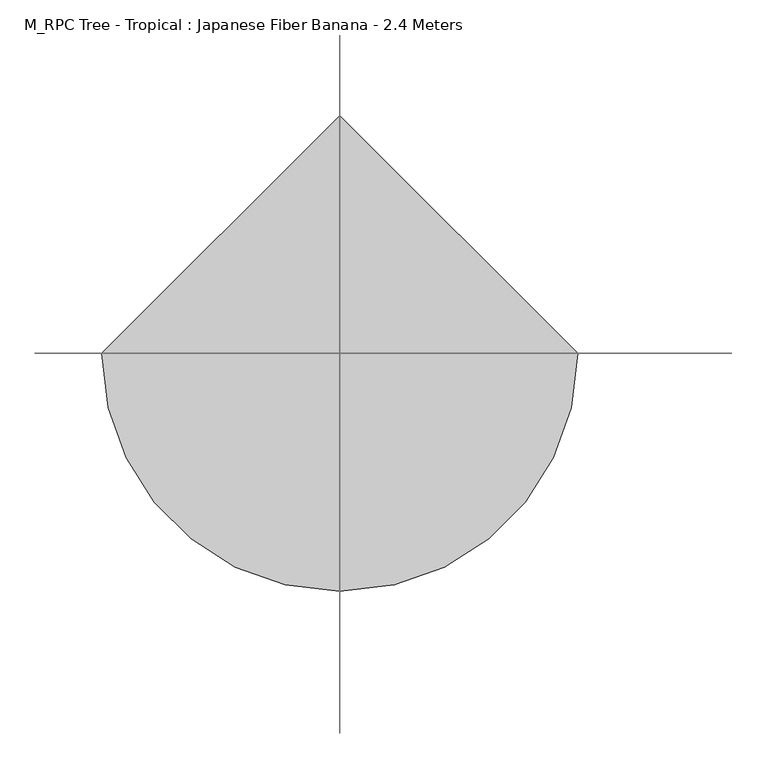
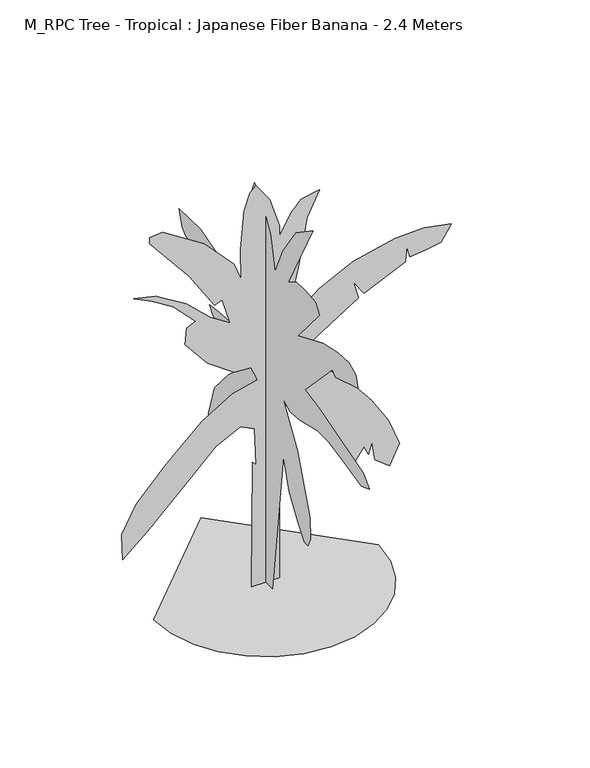
"""IFC4 building model written with IfcOpenShell, lengths in millimetres: geographic element geometry, M_RPC Tree - Tropical : Japanese Fiber Banana - 2.4 Meters."""

from ifc_helpers import new_model, si_unit, origin, place, context, project, spatial, triangles, source, transform, mapped, element, save


def m_rpc_tree_tropical_japanese_fiber_banana_2_4_meters_2e6d15ad(model_context):
    return source(origin(), model_context, "Body", "Tessellation", [
        triangles([(-639.3178808, 0.0, 3.7e-06), (-622.4128807, -146.5347148, 3.7e-06), (-574.2626584, -281.1033905, 3.7e-06), (-498.7249, -399.8512839, 3.7e-06), (-399.6546026, -498.9215813, 3.7e-06), (-280.9067273, -574.4593397, 3.7e-06), (-146.3380426, -622.6095257, 3.7e-06), (0.196699, -639.5145258, 3.7e-06), (146.7313871, -622.6095257, 3.7e-06), (281.3000536, -574.4593397, 3.7e-06), (400.0479652, -498.9215813, 3.7e-06), (499.1182626, -399.8512839, 3.7e-06), (574.656021, -281.1033905, 3.7e-06), (622.8061707, -146.5344696, 3.7e-06), (639.7111708, 5.59e-05, 3.7e-06), (0.1965872, 639.5145258, 3.7e-06), (72.5559047, -2.4e-06, 1465.492234), (85.0391952, -3.9e-06, 1478.3097656), (106.8852636, -6.2e-06, 1497.8148251), (136.5331088, -9.2e-06, 1522.8923641), (172.4227059, -1.28e-05, 1552.4299507), (212.9935943, -1.67e-05, 1585.3100658), (256.6849863, -2.09e-05, 1620.4176613), (301.9376202, -2.52e-05, 1656.6427757), (497.3357769, -3.68e-05, 1754.3430622), (735.2139896, -4.34e-05, 1809.5632381), (900.8770609, -4.39e-05, 1813.8107986), (1053.7975233, -4.04e-05, 1784.075695), (994.3298595, -2.97e-05, 1694.872855), (909.3720366, -2.77e-05, 1677.8804329), (820.1692692, -2.67e-05, 1669.3853119), (803.1767017, -3.43e-05, 1733.1030796), (794.6816534, -2.42e-05, 1648.1478001), (556.8059478, -1.15e-05, 1541.9523926), (497.3357769, -2.16e-05, 1626.9076721), (527.0708805, -9.5e-06, 1524.9598251), (246.7159545, 1.13e-05, 1350.8018509), (204.2378242, 1.99e-05, 1278.5891075), (450.610613, 4.47e-05, 1070.4459257), (599.2835876, 6.7e-05, 883.5427992), (696.9839104, 8.52e-05, 730.6223368), (760.699062, 0.0001045, 569.2043189), (701.2313982, 0.0001181, 454.5139721), (620.5211357, 0.0001105, 518.2316671), (603.5311117, 9.74e-05, 628.6744898), (582.2910564, 0.000105, 564.9567947), (556.8059478, 9.84e-05, 620.1795141), (510.0808202, 0.0001065, 552.2142586), (233.9724192, 6.75e-05, 879.2953114), (98.0427347, 4.83e-05, 1040.7108221), (81.0516842, 4.01e-05, 1108.6760777), (76.8036695, 0.0001723, 0.0), (-80.3648348, 0.0001723, 0.0), (-76.1170745, 8.32e-05, 747.6123608), (-54.8780048, 8.57e-05, 726.3748489), (-63.3737798, 5.99e-05, 943.0130064), (-144.0820393, 5.48e-05, 985.4906462), (-284.259248, 6.29e-05, 917.5254633), (-492.4023934, 8.72e-05, 713.6297693), (-675.0579958, 0.000108, 539.4717224), (-815.2334513, 0.0001222, 420.5313443), (-819.4834826, 0.000104, 573.4543502), (-738.7732201, 8.57e-05, 726.3748489), (-564.6151368, 6.39e-05, 909.030415), (-364.9670033, 4.22e-05, 1091.685981), (-190.8077029, 2.95e-05, 1197.878845), (-46.382475, 2.55e-05, 1231.8614365), (-84.6125952, 1.53e-05, 1316.8191868), (-182.312164, 1.43e-05, 1325.3143078), (-330.9843756, 1.7e-06, 1431.5095699), (-458.419802, -1.71e-05, 1588.6775928), (-449.9247537, -2.82e-05, 1682.1278481), (-398.9495948, -3.13e-05, 1707.6155365), (-526.3850212, -4.69e-05, 1839.2983418), (-649.5704527, -5.61e-05, 1915.7586456), (-751.518227, -6.21e-05, 1966.7312611), (-628.3303974, -5.86e-05, 1936.9961575), (-454.1722778, -4.59e-05, 1830.8033661), (-318.2418394, -3.07e-05, 1703.367976), (-203.5512383, -2.21e-05, 1631.1552326), (-250.2766384, -4.04e-05, 1784.075695), (-292.7542781, -3.83e-05, 1767.0855984), (-437.1797104, -6.52e-05, 1992.2188042), (-662.3129889, -9.76e-05, 2264.0772102), (-662.3129889, -0.0001021, 2302.3074348), (-585.852685, -0.0001027, 2306.55485), (-352.2244308, -8.49e-05, 2157.8819481), (-182.312164, -6.32e-05, 1975.2263821), (-139.8340246, -5.05e-05, 1869.0334454), (-144.0820393, -7.18e-05, 2047.4389801), (-122.8429742, -9.86e-05, 2272.574802), (-88.8603646, -0.0001102, 2370.2726177), (-54.8780048, -0.0001138, 2400.0077213), (21.5823377, -0.0001011, 2293.8123138), (76.8036695, -7.99e-05, 2115.4043083), (76.8036695, -7.28e-05, 2055.9365719), (144.7686344, -8.64e-05, 2170.626955), (199.9900457, -9.35e-05, 2230.0946915), (306.1851625, -9.61e-05, 2251.3346741), (233.9724192, -7.89e-05, 2106.9091873), (187.2465104, -4.8e-05, 1847.7934628), (140.5208741, -2.26e-05, 1635.4027931), (122.4893166, -1.78e-05, 1594.7825981), (105.4982571, -1.32e-05, 1556.205011), (90.5874576, -9.1e-06, 1521.7148197), (78.7976703, -5.7e-06, 1493.3547775), (71.1688981, -3.3e-06, 1473.1696724), (68.7416435, -2.1e-06, 1463.1996414), (0.1966114, -224.793728, 1941.5012604), (0.1966075, -300.4359677, 1984.7263836), (0.1966072, -390.4887377, 1988.3263092), (0.1966081, -487.7415587, 1977.5213001), (0.196613, -527.3641766, 1923.4911678), (0.1966355, -314.8460074, 1671.3478374), (0.1966262, -559.7842907, 1775.8081764), (0.1966233, -707.4672821, 1808.2258198), (0.196623, -815.5276194, 1811.8283615), (0.1966255, -887.570315, 1783.0106438), (0.1966316, -905.5804075, 1714.5729607), (0.1966378, -685.8547205, 1646.1328068), (0.1966352, -657.0396189, 1674.9503792), (0.1966606, -386.8862323, 1390.3894054), (0.1966629, -516.5591675, 1365.1743748), (0.1966745, -959.6105398, 1235.5014759), (0.1966796, -1020.8457556, 1177.8688019), (0.1966822, -941.6005199, 1149.0511568), (0.1966796, -808.3250793, 1177.8688019), (0.1966761, -613.8144957, 1217.4913834), (0.1966761, -509.3541203, 1217.4913834), (0.1966796, -336.4560619, 1177.8688019), (0.1966806, -242.8040204, 1167.0612494), (0.1966774, -167.1610358, 1203.0813618), (0.1966973, -311.243502, 979.7556038), (0.1967267, -433.7113901, 651.9695795), (0.1967379, -440.9164009, 525.899186), (0.1967428, -415.7013339, 471.8665103), (0.1967428, -379.6812215, 471.8665103), (0.1967353, -318.4460057, 554.7142877), (0.1967234, -228.3957247, 687.9896919), (0.196708, -174.3650655, 860.8877867), (0.1967286, -145.5487194, 630.3570179), (0.196785, -66.3037109, 3.7e-06), (0.196785, 81.3800072, 3.7e-06), (0.1967656, 81.3800072, 216.1224368), (0.1967721, 63.3697012, 144.0817123), (0.1967482, 34.5533597, 410.6338017), (0.1967202, 34.5533597, 724.0098043), (0.1966945, 77.7777471, 1012.1732471), (0.1966986, 171.4310513, 965.348053), (0.1967118, 326.3185266, 817.6625908), (0.1967222, 423.5738548, 702.3972427), (0.1967286, 437.9814056, 630.3570179), (0.196726, 463.1964726, 659.1745903), (0.1967334, 459.5939672, 576.3268493), (0.1967302, 520.829183, 612.3469254), (0.196735, 542.4417446, 558.3167931), (0.1967247, 564.0543062, 673.5821411), (0.196708, 506.4216322, 860.8877867), (0.1966935, 369.5436862, 1022.9807997), (0.1966771, 167.8290364, 1206.6838308), (0.1966729, 268.6858526, 1253.5115685), (0.19667, 387.5537424, 1285.9290665), (0.1966713, 452.3914636, 1271.5215157), (0.19667, 520.829183, 1285.9290665), (0.1966661, 556.8492954, 1329.1541897), (0.1966648, 459.5939672, 1343.5617405), (0.1966635, 250.6757964, 1357.9692913), (0.1966581, 326.3185266, 1419.2045071), (0.1966465, 506.4216322, 1548.8774059), (0.196642, 718.9423084, 1599.3076126), (0.196642, 787.3799915, 1599.3076126), (0.1966387, 827.0026457, 1635.3277977), (0.1966307, 855.8202181, 1725.3779697), (0.1966304, 643.2995419, 1728.9805115), (0.1966358, 434.3789002, 1667.7452957), (0.1966413, 279.493387, 1606.51008), (0.1966552, 106.5943384, 1451.6221504), (0.1966184, 149.8187259, 1862.2559521), (0.1965917, 182.2370778, 2161.2244766), (0.1965763, 110.1963533, 2334.1224987), (0.1965824, 45.359645, 2265.6848156), (0.1965956, -44.6916443, 2118.0018242), (0.1966133, -87.9160272, 1919.8886261), (0.1965978, -167.1610358, 2092.7866482), (0.1965811, -296.8334441, 2280.0923664), (0.1965711, -462.5289625, 2391.7551727)], [[15, 16, 1], [14, 15, 1], [14, 1, 2], [13, 14, 2], [13, 2, 3], [13, 3, 4], [12, 13, 4], [11, 12, 4], [11, 4, 5], [11, 5, 6], [11, 6, 7], [11, 7, 8], [11, 8, 9], [11, 9, 10], [75, 76, 77], [45, 46, 47], [53, 54, 55], [60, 61, 62], [98, 99, 100], [97, 98, 100], [27, 28, 29], [27, 29, 30], [47, 48, 49], [60, 62, 63], [59, 60, 63], [59, 63, 64], [58, 59, 64], [58, 64, 65], [74, 75, 77], [74, 77, 78], [73, 74, 78], [73, 78, 79], [42, 43, 44], [42, 44, 45], [41, 42, 45], [92, 93, 94], [91, 92, 94], [96, 97, 100], [96, 100, 101], [52, 53, 55], [51, 52, 55], [51, 55, 56], [57, 58, 65], [57, 65, 66], [57, 66, 67], [27, 30, 31], [27, 31, 32], [26, 27, 32], [84, 85, 86], [83, 84, 86], [83, 86, 87], [83, 87, 88], [82, 83, 88], [81, 82, 88], [81, 88, 89], [56, 57, 67], [51, 56, 67], [91, 94, 95], [90, 91, 95], [90, 95, 96], [89, 90, 96], [89, 96, 101], [89, 101, 102], [33, 34, 35], [32, 33, 35], [26, 32, 35], [25, 26, 35], [24, 25, 35], [81, 89, 102], [80, 81, 102], [80, 102, 103], [80, 103, 104], [80, 104, 105], [80, 105, 106], [80, 106, 107], [40, 41, 45], [40, 45, 47], [40, 47, 49], [39, 40, 49], [38, 39, 49], [38, 49, 50], [38, 50, 51], [38, 51, 67], [38, 67, 68], [35, 36, 37], [24, 35, 37], [23, 24, 37], [22, 23, 37], [21, 22, 37], [20, 21, 37], [19, 20, 37], [18, 19, 37], [17, 18, 37], [17, 37, 38], [17, 38, 68], [108, 17, 68], [80, 107, 108], [80, 108, 68], [80, 68, 69], [80, 69, 70], [80, 70, 71], [79, 80, 71], [73, 79, 71], [73, 71, 72], [143, 144, 145], [185, 186, 109], [184, 185, 109], [155, 156, 157], [183, 184, 109], [151, 152, 153], [153, 154, 155], [164, 165, 166], [163, 164, 166], [124, 125, 126], [179, 180, 181], [172, 173, 174], [171, 172, 174], [170, 171, 174], [169, 170, 174], [169, 174, 175], [142, 143, 145], [141, 142, 145], [141, 145, 146], [141, 146, 147], [140, 141, 147], [140, 147, 148], [162, 163, 166], [162, 166, 167], [161, 162, 167], [179, 181, 182], [178, 179, 182], [178, 182, 183], [153, 155, 157], [153, 157, 158], [151, 153, 158], [150, 151, 158], [150, 158, 159], [149, 150, 159], [149, 159, 160], [148, 149, 160], [124, 126, 127], [123, 124, 127], [123, 127, 128], [123, 128, 129], [118, 119, 120], [117, 118, 120], [116, 117, 120], [116, 120, 121], [115, 116, 121], [115, 121, 122], [114, 115, 122], [168, 169, 175], [168, 175, 176], [168, 176, 177], [167, 168, 177], [177, 178, 183], [122, 123, 129], [122, 129, 130], [112, 113, 114], [111, 112, 114], [110, 111, 114], [109, 110, 114], [183, 109, 114], [177, 183, 114], [177, 114, 122], [177, 122, 130], [177, 130, 131], [177, 131, 132], [167, 177, 132], [161, 167, 132], [160, 161, 132], [148, 160, 132], [140, 148, 132], [140, 132, 133], [140, 133, 134], [139, 140, 134], [138, 139, 134], [138, 134, 135], [137, 138, 135], [137, 135, 136]], closed=False),
    ])


if __name__ == "__main__":
    model = new_model("IFC4")
    model_context = context("Model", 3, world=origin())
    ifc_project = project(units=[si_unit("LENGTHUNIT", "METRE", prefix="MILLI")], contexts=[model_context])
    site = spatial("IfcSite", under=ifc_project)
    building = spatial("IfcBuilding", under=site)
    placement = place(None, origin())
    m_rpc_tree_tropical_japanese_fiber_banana_2_4_meters_shape = m_rpc_tree_tropical_japanese_fiber_banana_2_4_meters_2e6d15ad(model_context)
    element("IfcGeographicElement", 1, ObjectType="M_RPC Tree - Tropical : Japanese Fiber Banana - 2.4 Meters", at=placement, inside=building, context=model_context, shape_type="MappedRepresentation", body=[
        mapped(m_rpc_tree_tropical_japanese_fiber_banana_2_4_meters_shape, transform((0.0, 0.0, 0.0), x_axis=(1.0, 0.0, 0.0), y_axis=(0.0, 1.0, 0.0), z_axis=(0.0, 0.0, 1.0))),
    ])
    save(model, "model.ifc")

# Revit data of these elements
# Type "M_RPC Tree - Tropical : Japanese Fiber Banana - 2.4 Meters"
#   built-in parameter 1005198 = "{2, 15},{39, RPC-16-FVGT-NR7X-7G1M-A000-ST1L-LVER-AU},{1, 0},{1, 0},{2, 35},{1, 8},{5, Color},{1, 0},{1, 0},{3, 0.8},{3, 0.8},{3, 0.8},{1, 8},{7, BBoxMin},{1, 0},{1, 0},{1, 0},{1, 0},{1, 0},{1, 8},{7, BBoxMax},{1, 0},{1, 0},{1, 0},{1, 0},{1, 0},{2, 11},{9, RPCTypeId},{1, 0},{1, 0},{39, RPC-16-FVGT-NR7X-7G1M-A000-ST1L-LVER-AU},{1, 6},{14, RPCPlantHeight},{1, 0},{1, 0},{7, 7.87402},{2, 11},{7, keyword},{1, 0},{1, 0},{62, :Geometry:RPC:Japanese Fiber Banana:Musa basjoo:Tree:Tropical.},{2, 11},{8, category},{1, 0},{1, 0},{17, :Trees [Tropical]},{2, 11},{12, LocalizedUID},{1, 0},{1, 0},{21, Japanese Fiber Banana},{2, 14},{6, Height},{1, 0},{1, 0},{7, 7.87402},{1, 2},{16, Cast Reflections},{1, 0},{1, 0},{1, 0},{1, 2},{12, Cast Shadows},{1, 0},{1, 0},{1, 1},{1, 2},{9, Lock View},{1, 0},{1, 0},{1, 0},{1, 4},{5, ViewC},{1, 0},{1, 0},{1, 0},{2, 11},{20, AdvancedUIDefinition},{1, 0},{1, 0},{0, },{2, 11},{10, AssetLibID},{1, 0},{1, 0},{36, 4D3F6E72-3F99-4203-98E9-AF80B3C7A7A4},{2, 11},{10, BaseSchema},{1, 0},{1, 0},{9, RPCSchema},{2, 11},{12, ExchangeGUID},{1, 0},{1, 0},{0, },{1, 2},{6, Hidden},{1, 0},{1, 0},{1, 0},{1, 4},{11, RPCCategory},{1, 0},{1, 0},{1, 0},{2, 11},{8, RPCImage},{1, 0},{1, 0},{0, },{1, 4},{13, SchemaVersion},{1, 0},{1, 0},{1, 4},{2, 11},{12, UIDefinition},{1, 0},{1, 0},{0, },{2, 11},{6, UIName},{1, 0},{1, 0},{39, RPC-16-FVGT-NR7X-7G1M-A000-ST1L-LVER-AU},{2, 11},{11, VersionGUID},{1, 0},{1, 0},{9, RPCSchema},{2, 11},{9, assettype},{1, 0},{1, 0},{11, RPCGeometry},{2, 11},{11, description},{1, 0},{1, 0},{0, },{2, 11},{9, localname},{1, 0},{1, 0},{3, RPC},{2, 11},{9, localtype},{1, 0},{1, 0},{3, RPC},{1, 4},{8, revision},{1, 0},{1, 0},{1, 1},{2, 11},{9, thumbnail},{1, 0},{1, 0},{0, },{1, 4},{7, version},{1, 0},{1, 0},{1, 1},{1, 2},{20, RPC_Cast Reflections},{1, 0},{1, 0},{1, 1},{1, 2},{16, RPC_Cast Shadows},{1, 0},{1, 0},{1, 1},{1, 2},{13, RPC_Lock View},{1, 0},{1, 0},{1, 0},{1, 4},{9, RPC_ViewC},{1, 0},{1, 0},{1, 0},{21, assetlibrary_base.fbx},{1, 5},"
#   built-in parameter 1005195 = "RPC-16-FVGT-NR7X-7G1M-A000-ST1L-LVER-AU"
#   Type Comments = "Japanese Fiber Banana"
#   Height = 2400 mm
#   Plan Symbol = element 405753
#   Description = (empty or 0)
#   Default Elevation = 0
